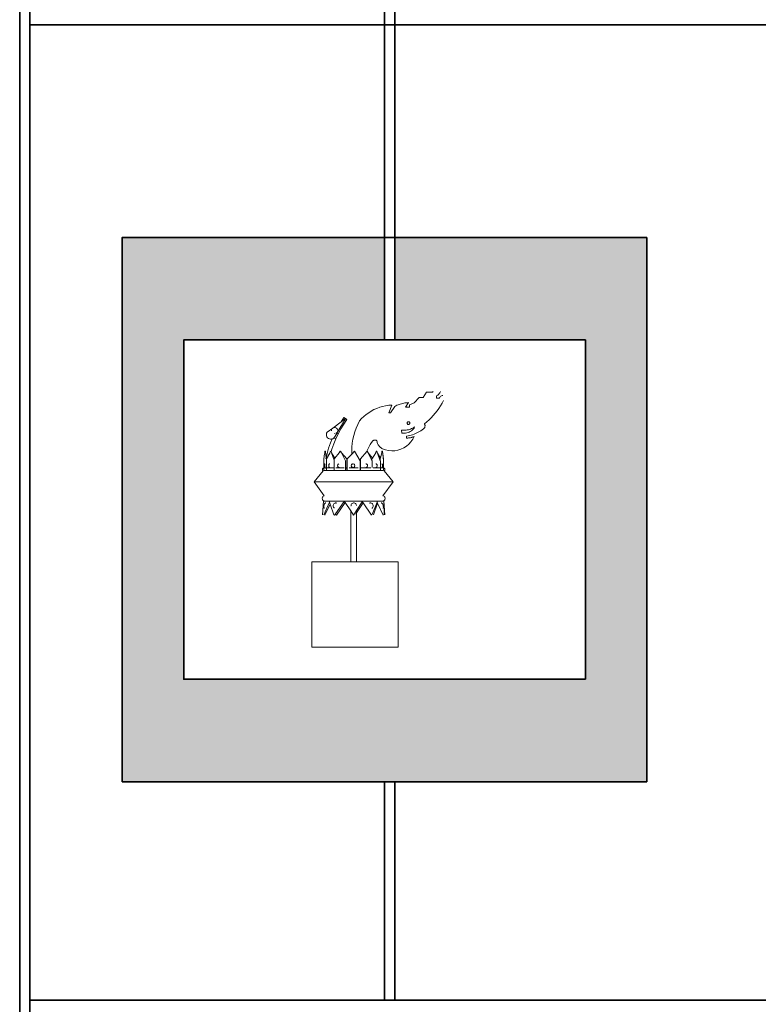
# Model space of a CAD drawing. Units: millimetres. Extents: x 2322 to 2394, y 1600 to 1790.
# Tile 2 of 5: x 2322 to 2358, y 1648 to 1696. Entities that reach past the tile are written whole.
import ezdxf

# ---------------------------------------------------------------- set-up
doc = ezdxf.new("R2010")
doc.units = ezdxf.units.MM
for name, color, linetype, lineweight in [('A-FURN', 7, 'Continuous', 35), ('A-FURN-ACCS', 8, 'Continuous', 18), ('A-FURN-PATT', 18, 'Continuous', 13)]:
    doc.layers.add(name, color=color, linetype=linetype, lineweight=lineweight)

msp = doc.modelspace()

# ---------------------------------------------------------------- hatches: boundary and pattern name
at = {"layer": 'A-FURN-PATT'}
h = msp.add_hatch(color=256, dxfattribs=at)
h.dxf.hatch_style = 1
h.paths.add_polyline_path([(2392.874, 1742.691), (2367.299, 1742.691), (2367.299, 1716.15), (2378.094, 1716.15), (2378.094, 1721.15), (2376.822, 1721.15), (2370.299, 1721.15), (2370.299, 1737.691), (2389.874, 1737.691), (2389.874, 1721.15), (2378.594, 1721.15), (2378.594, 1716.15), (2392.874, 1716.15)])
h.paths.add_polyline_path([(2352.154, 1685.571), (2339.867, 1685.571), (2339.867, 1680.571), (2349.154, 1680.571), (2349.154, 1664.029), (2329.579, 1664.029), (2329.579, 1680.571), (2339.367, 1680.571), (2339.367, 1685.571), (2326.579, 1685.571), (2326.579, 1659.029), (2352.154, 1659.029)])
h.paths.add_polyline_path([(2390.882, 1635.073), (2365.307, 1635.073), (2365.307, 1608.531), (2390.882, 1608.531)])
h.paths.add_polyline_path([(2387.882, 1630.073), (2387.882, 1613.531), (2368.307, 1613.531), (2368.307, 1630.073)], flags=16)
h.paths.add_polyline_path([(2373.463, 1622.711), (2373.46, 1622.644), (2373.462, 1622.642)], flags=0)
h.paths.add_polyline_path([(2380.387, 1618.619), (2380.387, 1618.619), (2380.35, 1618.619)], flags=0)
h.paths.add_polyline_path([(2377.431, 1618.132), (2377.363, 1618.141), (2377.19, 1618.152), (2377.145, 1618.149), (2376.982, 1618.132)], flags=0)
h.paths.add_polyline_path([(2376.126, 1618.152), (2375.767, 1618.152), (2375.734, 1618.152), (2375.734, 1618.152), (2375.028, 1618.152), (2375.028, 1618.198), (2374.578, 1618.295), (2374.235, 1618.449), (2373.926, 1618.69), (2373.709, 1619.163), (2373.66, 1619.336), (2373.672, 1619.402), (2373.73, 1620.54), (2373.702, 1622.038), (2373.678, 1622.131), (2373.705, 1621.917), (2373.73, 1620.54), (2373.667, 1619.311), (2373.709, 1619.163), (2373.87, 1618.812), (2373.949, 1618.699), (2374.037, 1618.604), (2374.187, 1618.486), (2374.3, 1618.42), (2374.485, 1618.337), (2374.688, 1618.272), (2374.979, 1618.209), (2375.028, 1618.203), (2375.028, 1618.372), (2375.028, 1618.619), (2377.125, 1618.619), (2377.165, 1620.356), (2377.172, 1620.356), (2377.172, 1620.357), (2377.341, 1620.357), (2377.354, 1620.357), (2377.354, 1623.532), (2377.38, 1623.766), (2377.629, 1623.72), (2377.726, 1623.72), (2377.722, 1623.891), (2377.719, 1624.041), (2377.644, 1624.123), (2377.631, 1624.228), (2377.644, 1624.211), (2377.677, 1624.213), (2377.688, 1624.153), (2377.757, 1624.059), (2377.78, 1623.72), (2377.883, 1623.72), (2378.152, 1623.76), (2378.155, 1620.358), (2378.298, 1620.356), (2378.301, 1620.356), (2378.362, 1620.357), (2378.402, 1618.619), (2377.354, 1618.619), (2377.125, 1618.619), (2375.028, 1618.619), (2375.028, 1618.372), (2375.028, 1618.177), (2375.049, 1618.152), (2375.734, 1618.152), (2375.756, 1618.153), (2375.767, 1618.152), (2376.126, 1618.152), (2376.144, 1618.154), (2376.168, 1618.151)], flags=0)
h.paths.add_polyline_path([(2380.5, 1618.343), (2380.401, 1618.342), (2380.5, 1618.342)], flags=0)
h.paths.add_polyline_path([(2378.836, 1627.111), (2378.86, 1627.114), (2378.771, 1627.114), (2378.773, 1627.108)], flags=0)
h.paths.add_polyline_path([(2378.972, 1627.091), (2379.09, 1626.957), (2378.972, 1626.879), (2378.964, 1626.862), (2378.975, 1626.787), (2379.128, 1626.434), (2379.25, 1626.246), (2379.42, 1626.03), (2379.646, 1625.791), (2380.15, 1625.354), (2380.519, 1624.956), (2380.743, 1624.553), (2380.884, 1624.119), (2380.94, 1623.673), (2380.977, 1621.652), (2380.892, 1619.98), (2380.807, 1619.502), (2380.712, 1619.163), (2380.621, 1618.942), (2380.422, 1618.619), (2380.413, 1618.619), (2380.386, 1618.619), (2380.474, 1618.703), (2380.621, 1618.942), (2380.712, 1619.163), (2380.807, 1619.502), (2380.892, 1619.98), (2380.977, 1621.652), (2380.94, 1623.673), (2380.9, 1623.987), (2380.843, 1624.244), (2380.778, 1624.446), (2380.693, 1624.644), (2380.585, 1624.839), (2380.452, 1625.029), (2380.15, 1625.354), (2379.646, 1625.791), (2379.324, 1626.132), (2379.128, 1626.434), (2378.92, 1626.915), (2378.841, 1626.975), (2378.869, 1626.811), (2379.027, 1626.915), (2379.041, 1626.939), (2379.037, 1626.997), (2379.02, 1627.036), (2378.879, 1627.196), (2378.841, 1627.151)], flags=0)
h.paths.add_polyline_path([(2375.501, 1627.114), (2375.642, 1627.103), (2375.561, 1626.855), (2375.555, 1626.827), (2375.48, 1626.868), (2375.292, 1626.434), (2375.097, 1626.132), (2374.775, 1625.791), (2374.271, 1625.354), (2374.13, 1625.216), (2373.969, 1625.029), (2373.836, 1624.839), (2373.728, 1624.644), (2373.643, 1624.446), (2373.537, 1624.119), (2373.52, 1623.987), (2373.601, 1624.348), (2373.773, 1624.748), (2374.034, 1625.122), (2374.271, 1625.354), (2374.775, 1625.791), (2375.001, 1626.03), (2375.171, 1626.246), (2375.292, 1626.434), (2375.445, 1626.787), (2375.447, 1626.797), (2375.334, 1627.042)], flags=0)
h.paths.add_polyline_path([(2375.398, 1627.114), (2375.384, 1626.997), (2375.411, 1627.054), (2375.531, 1627.169), (2375.597, 1627.114)], flags=0)
h.paths.add_polyline_path([(2377.985, 1623.628), (2377.785, 1623.645), (2377.786, 1623.634), (2377.764, 1623.634), (2377.729, 1623.636), (2377.728, 1623.656), (2377.701, 1623.664), (2377.421, 1623.752), (2377.412, 1623.748), (2377.629, 1623.72), (2377.78, 1623.72), (2377.783, 1623.68)], flags=0)
h.paths.add_polyline_path([(2377.348, 1620.357), (2377.335, 1620.357), (2377.327, 1620.356), (2377.354, 1620.356)], flags=0)
h.paths.add_polyline_path([(2377.834, 1620.357), (2377.854, 1620.356), (2377.911, 1620.356), (2377.923, 1620.357)], flags=0)
h.paths.add_polyline_path([(2378.155, 1620.356), (2378.155, 1620.356), (2378.014, 1620.356), (2378.002, 1620.357), (2377.96, 1620.356), (2377.956, 1620.356), (2377.923, 1620.357), (2378.111, 1620.357), (2378.119, 1620.356), (2378.144, 1620.356), (2378.163, 1620.357), (2378.163, 1620.357), (2378.157, 1620.357), (2378.149, 1620.356)], flags=0)
h.paths.add_polyline_path([(2377.609, 1620.357), (2377.623, 1620.356), (2377.653, 1620.357), (2377.738, 1620.356), (2377.743, 1620.357)], flags=0)
h.paths.add_polyline_path([(2380.479, 1618.152), (2380.406, 1618.152), (2380.313, 1618.151), (2380.107, 1618.152), (2380.104, 1618.152), (2380.108, 1618.151), (2379.961, 1618.152), (2379.793, 1618.152), (2377.32, 1618.152), (2377.3, 1618.149), (2377.253, 1618.152), (2379.793, 1618.152), (2380.01, 1618.153), (2380.21, 1618.152), (2380.229, 1618.152), (2380.231, 1618.152), (2380.394, 1618.152), (2380.48, 1618.152)], flags=0)

# ---------------------------------------------------------------- linework, layer by layer
at = {"layer": 'A-FURN'}
for p, q in [((2321.58, 1599.925), (2321.58, 1755.925)), ((2322.08, 1600.425), (2322.08, 1755.425)), ((2339.367, 1680.571), (2339.367, 1701.937)), ((2339.867, 1680.571), (2339.867, 1701.937)), ((2322.08, 1695.937), (2393.08, 1695.937)), ((2352.154, 1685.571), (2352.154, 1659.029)), ((2339.367, 1648.381), (2339.367, 1659.029)), ((2339.867, 1648.381), (2339.867, 1659.029)), ((2393.08, 1648.381), (2322.08, 1648.381))]:
    msp.add_line(p, q, dxfattribs=at)
msp.add_lwpolyline([(2352.154, 1659.029), (2326.579, 1659.029), (2326.579, 1685.571), (2352.154, 1685.571)], dxfattribs=at)
msp.add_lwpolyline([(2349.154, 1664.029), (2329.579, 1664.029), (2329.579, 1680.571), (2349.154, 1680.571)], close=True, dxfattribs=at)
at = {"layer": 'A-FURN-ACCS'}
for p, q in [((2341.248, 1677.774), (2341.407, 1678.032)), ((2341.407, 1678.032), (2341.702, 1678.032)), ((2341.702, 1678.032), (2341.729, 1678.056)), ((2341.931, 1677.862), (2341.9, 1677.844)), ((2341.9, 1677.844), (2341.9, 1677.731)), ((2341.96, 1677.883), (2341.931, 1677.862)), ((2341.987, 1677.906), (2341.96, 1677.883)), ((2342.011, 1677.931), (2341.987, 1677.906)), ((2342.033, 1677.959), (2342.011, 1677.931)), ((2342.053, 1677.989), (2342.033, 1677.959)), ((2342.069, 1678.021), (2342.053, 1677.989)), ((2342.083, 1678.053), (2342.069, 1678.021)), ((2342.088, 1677.805), (2342.113, 1677.826)), ((2342.113, 1677.826), (2342.139, 1677.844)), ((2342.139, 1677.844), (2342.168, 1677.859)), ((2342.168, 1677.859), (2342.198, 1677.871)), ((2339.27, 1677.331), (2339.416, 1677.364)), ((2339.416, 1677.364), (2339.565, 1677.387)), ((2339.565, 1677.387), (2339.714, 1677.399)), ((2339.714, 1677.399), (2339.567, 1677.027)), ((2339.66, 1677.027), (2339.857, 1677.336)), ((2339.857, 1677.336), (2339.91, 1677.362)), ((2339.91, 1677.362), (2339.964, 1677.386)), ((2339.964, 1677.386), (2340.019, 1677.408)), ((2340.019, 1677.408), (2340.074, 1677.428)), ((2340.074, 1677.428), (2340.13, 1677.446)), ((2340.13, 1677.446), (2340.187, 1677.462)), ((2340.187, 1677.462), (2340.244, 1677.477)), ((2340.244, 1677.477), (2340.302, 1677.489)), ((2340.302, 1677.489), (2340.36, 1677.499)), ((2340.36, 1677.499), (2340.419, 1677.506)), ((2340.536, 1677.516), (2340.391, 1677.289)), ((2340.419, 1677.506), (2340.478, 1677.512)), ((2340.478, 1677.512), (2340.536, 1677.516)), ((2340.585, 1677.415), (2340.8, 1677.501)), ((2340.585, 1677.289), (2340.585, 1677.415)), ((2340.8, 1677.501), (2341.05, 1677.774)), ((2341.05, 1677.774), (2341.248, 1677.774)), ((2341.9, 1677.731), (2342.026, 1677.731)), ((2342.092, 1677.362), (2342.011, 1677.238)), ((2342.026, 1677.731), (2342.044, 1677.757)), ((2342.044, 1677.757), (2342.065, 1677.782)), ((2342.065, 1677.782), (2342.088, 1677.805)), ((2342.167, 1677.489), (2342.092, 1677.362)), ((2342.236, 1677.619), (2342.167, 1677.489)), ((2338.354, 1676.84), (2338.469, 1676.936)), ((2338.469, 1676.936), (2338.59, 1677.024)), ((2338.59, 1677.024), (2338.717, 1677.104)), ((2338.717, 1677.104), (2338.849, 1677.174)), ((2338.849, 1677.174), (2338.986, 1677.236)), ((2338.986, 1677.236), (2339.126, 1677.288)), ((2339.126, 1677.288), (2339.27, 1677.331)), ((2339.567, 1677.027), (2339.66, 1677.027)), ((2340.391, 1677.289), (2340.585, 1677.289)), ((2341.737, 1676.89), (2341.636, 1676.783)), ((2341.834, 1677.002), (2341.737, 1676.89)), ((2341.925, 1677.118), (2341.834, 1677.002)), ((2342.011, 1677.238), (2341.925, 1677.118)), ((2337.246, 1676.583), (2336.842, 1676.278)), ((2337.456, 1676.729), (2337.044, 1676.028)), ((2337.231, 1676.236), (2337.371, 1676.467)), ((2337.386, 1676.787), (2337.246, 1676.583)), ((2337.456, 1676.74), (2337.246, 1676.583)), ((2337.371, 1676.467), (2337.525, 1676.692)), ((2337.456, 1676.74), (2337.386, 1676.787)), ((2337.456, 1676.729), (2337.456, 1676.74)), ((2337.525, 1676.692), (2337.456, 1676.74)), ((2338.058, 1676.454), (2337.982, 1676.279)), ((2338.144, 1676.625), (2338.058, 1676.454)), ((2338.144, 1676.625), (2338.245, 1676.736)), ((2338.245, 1676.736), (2338.354, 1676.84)), ((2340.462, 1676.529), (2340.466, 1676.546)), ((2340.462, 1676.512), (2340.462, 1676.529)), ((2340.466, 1676.495), (2340.462, 1676.512)), ((2340.466, 1676.546), (2340.475, 1676.561)), ((2340.475, 1676.479), (2340.466, 1676.495)), ((2340.475, 1676.561), (2340.488, 1676.574)), ((2340.487, 1676.467), (2340.475, 1676.479)), ((2340.502, 1676.458), (2340.487, 1676.467)), ((2340.488, 1676.574), (2340.503, 1676.582)), ((2340.519, 1676.453), (2340.502, 1676.458)), ((2340.503, 1676.582), (2340.52, 1676.587)), ((2340.537, 1676.453), (2340.519, 1676.453)), ((2340.52, 1676.587), (2340.538, 1676.587)), ((2340.554, 1676.458), (2340.537, 1676.453)), ((2340.538, 1676.587), (2340.555, 1676.582)), ((2340.569, 1676.467), (2340.554, 1676.458)), ((2340.555, 1676.582), (2340.57, 1676.573)), ((2340.582, 1676.479), (2340.569, 1676.467)), ((2340.57, 1676.573), (2340.582, 1676.561)), ((2340.582, 1676.561), (2340.591, 1676.546)), ((2340.591, 1676.494), (2340.582, 1676.479)), ((2340.591, 1676.546), (2340.595, 1676.529)), ((2340.595, 1676.511), (2340.591, 1676.494)), ((2340.595, 1676.529), (2340.595, 1676.511)), ((2341.42, 1676.582), (2341.305, 1676.489)), ((2341.305, 1676.489), (2341.317, 1676.469)), ((2341.317, 1676.469), (2341.326, 1676.447)), ((2341.326, 1676.447), (2341.332, 1676.425)), ((2341.332, 1676.425), (2341.336, 1676.401)), ((2341.336, 1676.378), (2341.334, 1676.354)), ((2341.336, 1676.401), (2341.336, 1676.378)), ((2341.53, 1676.68), (2341.42, 1676.582)), ((2341.636, 1676.783), (2341.53, 1676.68)), ((2336.539, 1676.023), (2336.529, 1675.969)), ((2336.529, 1675.958), (2336.529, 1675.969)), ((2336.529, 1675.958), (2336.533, 1675.903)), ((2336.533, 1675.903), (2336.552, 1675.851)), ((2336.564, 1676.073), (2336.539, 1676.023)), ((2336.842, 1676.278), (2336.564, 1676.073)), ((2336.778, 1676.15), (2336.78, 1676.187)), ((2336.778, 1676.149), (2336.778, 1676.15)), ((2336.778, 1676.143), (2336.778, 1676.149)), ((2336.78, 1676.187), (2336.792, 1676.222)), ((2336.792, 1676.222), (2336.813, 1676.253)), ((2336.813, 1676.253), (2336.842, 1676.278)), ((2336.842, 1676.278), (2336.876, 1676.295)), ((2336.876, 1676.295), (2336.913, 1676.303)), ((2336.913, 1676.303), (2336.952, 1676.301)), ((2336.927, 1676.02), (2336.924, 1676.013)), ((2337.039, 1676.018), (2336.929, 1675.831)), ((2336.952, 1676.301), (2336.988, 1676.289)), ((2336.988, 1676.289), (2337.021, 1676.269)), ((2336.989, 1675.755), (2337.099, 1675.989)), ((2336.996, 1676.038), (2337.003, 1676.034)), ((2337.015, 1676.043), (2337.01, 1676.045)), ((2337.021, 1676.269), (2337.046, 1676.242)), ((2337.044, 1676.028), (2337.039, 1676.018)), ((2337.099, 1675.989), (2337.039, 1676.018)), ((2337.044, 1676.028), (2337.103, 1675.998)), ((2337.046, 1676.242), (2337.064, 1676.208)), ((2337.064, 1676.208), (2337.072, 1676.172)), ((2337.071, 1676.167), (2337.072, 1676.172)), ((2337.071, 1676.167), (2337.072, 1676.166)), ((2337.231, 1676.236), (2337.103, 1675.998)), ((2337.865, 1675.915), (2337.823, 1675.729)), ((2337.918, 1676.099), (2337.865, 1675.915)), ((2337.982, 1676.279), (2337.918, 1676.099)), ((2340.245, 1676.169), (2340.189, 1676.174)), ((2340.189, 1676.174), (2340.203, 1676.034)), ((2340.264, 1676.025), (2340.203, 1676.034)), ((2340.302, 1676.167), (2340.245, 1676.169)), ((2340.326, 1676.023), (2340.264, 1676.025)), ((2340.358, 1676.169), (2340.302, 1676.167)), ((2340.388, 1676.028), (2340.326, 1676.023)), ((2340.414, 1676.174), (2340.358, 1676.169)), ((2340.449, 1676.038), (2340.388, 1676.028)), ((2340.469, 1676.183), (2340.414, 1676.174)), ((2340.51, 1675.895), (2340.435, 1675.882)), ((2340.508, 1676.056), (2340.449, 1676.038)), ((2340.524, 1676.194), (2340.469, 1676.183)), ((2340.566, 1676.079), (2340.508, 1676.056)), ((2340.584, 1675.911), (2340.51, 1675.895)), ((2340.578, 1676.209), (2340.524, 1676.194)), ((2340.62, 1676.108), (2340.566, 1676.079)), ((2340.632, 1676.227), (2340.578, 1676.209)), ((2340.657, 1675.931), (2340.584, 1675.911)), ((2340.671, 1676.143), (2340.62, 1676.108)), ((2340.684, 1676.248), (2340.632, 1676.227)), ((2340.73, 1675.953), (2340.657, 1675.931)), ((2340.718, 1676.183), (2340.671, 1676.143)), ((2340.735, 1676.272), (2340.684, 1676.248)), ((2340.761, 1676.228), (2340.718, 1676.183)), ((2340.801, 1675.978), (2340.73, 1675.953)), ((2340.784, 1676.3), (2340.735, 1676.272)), ((2340.799, 1676.277), (2340.761, 1676.228)), ((2340.831, 1676.33), (2340.784, 1676.3)), ((2340.831, 1676.33), (2340.799, 1676.277)), ((2340.871, 1676.007), (2340.801, 1675.978)), ((2340.941, 1676.038), (2340.871, 1676.007)), ((2341.008, 1676.072), (2340.941, 1676.038)), ((2341.074, 1676.109), (2341.008, 1676.072)), ((2341.139, 1676.149), (2341.074, 1676.109)), ((2341.202, 1676.191), (2341.139, 1676.149)), ((2341.263, 1676.236), (2341.202, 1676.191)), ((2341.281, 1676.252), (2341.263, 1676.236)), ((2341.296, 1676.269), (2341.281, 1676.252)), ((2341.31, 1676.288), (2341.296, 1676.269)), ((2341.32, 1676.309), (2341.31, 1676.288)), ((2341.329, 1676.331), (2341.32, 1676.309)), ((2341.334, 1676.354), (2341.329, 1676.331)), ((2336.552, 1675.851), (2336.584, 1675.806)), ((2336.584, 1675.806), (2336.627, 1675.77)), ((2336.627, 1675.77), (2336.678, 1675.746)), ((2336.729, 1675.562), (2336.639, 1675.298)), ((2336.678, 1675.746), (2336.734, 1675.736)), ((2336.803, 1675.744), (2336.729, 1675.562)), ((2336.734, 1675.736), (2336.791, 1675.74)), ((2336.791, 1675.74), (2336.803, 1675.744)), ((2336.799, 1675.248), (2336.887, 1675.503)), ((2336.803, 1675.744), (2336.845, 1675.758)), ((2336.808, 1675.756), (2336.803, 1675.744)), ((2336.845, 1675.758), (2336.892, 1675.789)), ((2336.887, 1675.503), (2336.988, 1675.754)), ((2336.888, 1675.797), (2336.896, 1675.794)), ((2336.892, 1675.789), (2336.896, 1675.794)), ((2336.899, 1675.797), (2336.893, 1675.8)), ((2336.896, 1675.794), (2336.899, 1675.797)), ((2336.896, 1675.794), (2336.988, 1675.754)), ((2336.899, 1675.797), (2336.929, 1675.831)), ((2336.899, 1675.797), (2336.989, 1675.755)), ((2336.913, 1675.791), (2336.911, 1675.787)), ((2336.941, 1675.851), (2336.913, 1675.791)), ((2337.792, 1675.54), (2337.774, 1675.35)), ((2337.823, 1675.729), (2337.792, 1675.54)), ((2338.665, 1675.474), (2338.608, 1675.378)), ((2338.729, 1675.565), (2338.665, 1675.474)), ((2338.8, 1675.65), (2338.729, 1675.565)), ((2338.813, 1675.663), (2338.8, 1675.65)), ((2338.828, 1675.673), (2338.813, 1675.663)), ((2338.843, 1675.681), (2338.828, 1675.673)), ((2338.86, 1675.687), (2338.843, 1675.681)), ((2338.877, 1675.691), (2338.86, 1675.687)), ((2338.895, 1675.692), (2338.877, 1675.691)), ((2338.913, 1675.691), (2338.895, 1675.692)), ((2338.93, 1675.687), (2338.913, 1675.691)), ((2338.947, 1675.681), (2338.93, 1675.687)), ((2338.963, 1675.673), (2338.947, 1675.681)), ((2338.977, 1675.663), (2338.963, 1675.673)), ((2338.99, 1675.65), (2338.977, 1675.663)), ((2338.996, 1675.609), (2338.99, 1675.65)), ((2339.006, 1675.569), (2338.996, 1675.609)), ((2339.019, 1675.53), (2339.006, 1675.569)), ((2339.035, 1675.492), (2339.019, 1675.53)), ((2339.055, 1675.455), (2339.035, 1675.492)), ((2339.078, 1675.42), (2339.055, 1675.455)), ((2339.104, 1675.388), (2339.078, 1675.42)), ((2340.546, 1675.489), (2340.43, 1675.39)), ((2340.435, 1675.882), (2340.435, 1675.785)), ((2340.435, 1675.785), (2340.467, 1675.787)), ((2340.467, 1675.787), (2340.498, 1675.789)), ((2340.498, 1675.789), (2340.53, 1675.793)), ((2340.53, 1675.793), (2340.561, 1675.797)), ((2340.649, 1675.602), (2340.546, 1675.489)), ((2340.561, 1675.797), (2340.593, 1675.802)), ((2340.593, 1675.802), (2340.624, 1675.808)), ((2340.624, 1675.808), (2340.655, 1675.815)), ((2340.736, 1675.728), (2340.649, 1675.602)), ((2340.655, 1675.815), (2340.685, 1675.823)), ((2340.685, 1675.823), (2340.716, 1675.832)), ((2340.716, 1675.832), (2340.746, 1675.842)), ((2340.806, 1675.864), (2340.736, 1675.728)), ((2340.746, 1675.842), (2340.776, 1675.852)), ((2340.776, 1675.852), (2340.806, 1675.864)), ((2336.443, 1675.02), (2336.398, 1674.769)), ((2336.443, 1675.02), (2336.446, 1675.046)), ((2336.446, 1675.046), (2336.459, 1675.151)), ((2336.466, 1675.151), (2336.446, 1675.046)), ((2336.466, 1675.151), (2336.459, 1675.151)), ((2336.466, 1675.151), (2336.483, 1675.151)), ((2336.489, 1675.091), (2336.483, 1675.151)), ((2336.489, 1675.091), (2336.532, 1674.894)), ((2336.516, 1674.826), (2336.489, 1675.091)), ((2336.693, 1675.06), (2336.527, 1674.769)), ((2336.562, 1675.029), (2336.532, 1674.894)), ((2336.639, 1675.298), (2336.562, 1675.029)), ((2336.644, 1675.008), (2336.631, 1674.952)), ((2336.693, 1675.06), (2336.724, 1675.151)), ((2336.744, 1675.151), (2336.693, 1675.06)), ((2336.728, 1675.151), (2336.724, 1675.151)), ((2336.757, 1675.151), (2336.744, 1675.151)), ((2336.765, 1675.127), (2336.757, 1675.151)), ((2336.765, 1675.127), (2336.799, 1675.248)), ((2336.782, 1675.075), (2336.765, 1675.127)), ((2336.782, 1675.075), (2336.94, 1674.813)), ((2336.903, 1674.708), (2336.782, 1675.075)), ((2337.15, 1675.066), (2336.94, 1674.813)), ((2337.15, 1675.066), (2337.192, 1675.151)), ((2337.21, 1675.138), (2337.15, 1675.066)), ((2337.199, 1675.151), (2337.192, 1675.151)), ((2337.199, 1675.151), (2337.21, 1675.138)), ((2337.221, 1675.151), (2337.21, 1675.138)), ((2337.229, 1675.151), (2337.221, 1675.151)), ((2337.267, 1675.071), (2337.229, 1675.151)), ((2337.249, 1675.093), (2337.267, 1675.071)), ((2337.267, 1675.071), (2337.525, 1674.769)), ((2337.46, 1674.671), (2337.267, 1675.071)), ((2337.771, 1675.009), (2337.543, 1674.769)), ((2337.774, 1675.35), (2337.767, 1675.159)), ((2337.767, 1675.159), (2337.771, 1675.009)), ((2337.905, 1675.151), (2337.771, 1675.009)), ((2338.168, 1674.671), (2337.905, 1675.151)), ((2338.506, 1675.137), (2338.19, 1674.769)), ((2338.506, 1675.137), (2338.503, 1675.127)), ((2338.507, 1675.14), (2338.506, 1675.137)), ((2338.506, 1675.137), (2338.509, 1675.134)), ((2338.517, 1675.175), (2338.507, 1675.14)), ((2338.516, 1675.151), (2338.507, 1675.14)), ((2338.516, 1675.151), (2338.523, 1675.151)), ((2338.559, 1675.278), (2338.517, 1675.175)), ((2338.565, 1675.066), (2338.523, 1675.151)), ((2338.608, 1675.378), (2338.559, 1675.278)), ((2338.565, 1675.066), (2338.776, 1674.813)), ((2338.565, 1675.066), (2338.749, 1674.693)), ((2338.933, 1675.075), (2338.776, 1674.813)), ((2338.933, 1675.075), (2338.958, 1675.151)), ((2338.975, 1675.145), (2338.933, 1675.075)), ((2338.958, 1675.151), (2338.971, 1675.151)), ((2338.971, 1675.151), (2338.975, 1675.145)), ((2338.978, 1675.151), (2338.975, 1675.145)), ((2338.978, 1675.151), (2338.991, 1675.151)), ((2339.023, 1675.06), (2338.991, 1675.151)), ((2339.023, 1675.06), (2339.165, 1674.81)), ((2339.023, 1675.06), (2339.156, 1674.677)), ((2339.132, 1675.358), (2339.104, 1675.388)), ((2339.163, 1675.33), (2339.132, 1675.358)), ((2339.196, 1675.306), (2339.163, 1675.33)), ((2339.226, 1675.091), (2339.165, 1674.81)), ((2339.232, 1675.284), (2339.196, 1675.306)), ((2339.226, 1675.091), (2339.233, 1675.151)), ((2339.239, 1675.151), (2339.226, 1675.091)), ((2339.269, 1675.265), (2339.232, 1675.284)), ((2339.233, 1675.151), (2339.239, 1675.151)), ((2339.239, 1675.151), (2339.256, 1675.151)), ((2339.256, 1675.151), (2339.273, 1675.02)), ((2339.412, 1675.212), (2339.269, 1675.265)), ((2339.273, 1675.02), (2339.317, 1674.769)), ((2339.317, 1674.671), (2339.273, 1675.02)), ((2339.561, 1675.178), (2339.412, 1675.212)), ((2339.713, 1675.165), (2339.561, 1675.178)), ((2339.866, 1675.171), (2339.713, 1675.165)), ((2340.017, 1675.197), (2339.866, 1675.171)), ((2340.162, 1675.243), (2340.017, 1675.197)), ((2340.301, 1675.308), (2340.162, 1675.243)), ((2340.43, 1675.39), (2340.301, 1675.308)), ((2336.398, 1674.769), (2336.399, 1674.677)), ((2336.398, 1674.671), (2336.399, 1674.677)), ((2336.398, 1674.671), (2336.398, 1674.329)), ((2336.427, 1674.456), (2336.428, 1674.477)), ((2336.427, 1674.434), (2336.427, 1674.456)), ((2336.428, 1674.477), (2336.431, 1674.496)), ((2336.431, 1674.496), (2336.433, 1674.512)), ((2336.433, 1674.512), (2336.437, 1674.523)), ((2336.436, 1674.456), (2336.437, 1674.477)), ((2336.436, 1674.434), (2336.436, 1674.456)), ((2336.437, 1674.523), (2336.441, 1674.528)), ((2336.437, 1674.477), (2336.439, 1674.496)), ((2336.439, 1674.496), (2336.442, 1674.512)), ((2336.449, 1674.528), (2336.441, 1674.528)), ((2336.442, 1674.512), (2336.445, 1674.523)), ((2336.445, 1674.523), (2336.449, 1674.528)), ((2336.451, 1674.477), (2336.45, 1674.456)), ((2336.45, 1674.456), (2336.45, 1674.434)), ((2336.454, 1674.496), (2336.451, 1674.477)), ((2336.454, 1674.481), (2336.451, 1674.477)), ((2336.457, 1674.512), (2336.454, 1674.496)), ((2336.454, 1674.496), (2336.454, 1674.481)), ((2336.459, 1674.517), (2336.457, 1674.512)), ((2336.46, 1674.515), (2336.457, 1674.512)), ((2336.459, 1674.477), (2336.458, 1674.456)), ((2336.458, 1674.456), (2336.458, 1674.434)), ((2336.462, 1674.496), (2336.459, 1674.477)), ((2336.463, 1674.501), (2336.462, 1674.496)), ((2336.516, 1674.826), (2336.505, 1674.776)), ((2336.532, 1674.894), (2336.516, 1674.826)), ((2336.527, 1674.719), (2336.516, 1674.826)), ((2336.527, 1674.769), (2336.527, 1674.719)), ((2336.527, 1674.719), (2336.527, 1674.33)), ((2336.532, 1674.894), (2336.544, 1674.838)), ((2336.641, 1674.456), (2336.644, 1674.477)), ((2336.641, 1674.434), (2336.641, 1674.456)), ((2336.644, 1674.477), (2336.651, 1674.496)), ((2336.651, 1674.496), (2336.66, 1674.512)), ((2336.66, 1674.512), (2336.671, 1674.523)), ((2336.671, 1674.523), (2336.684, 1674.528)), ((2336.691, 1674.528), (2336.684, 1674.528)), ((2336.94, 1674.813), (2336.903, 1674.769)), ((2336.903, 1674.769), (2336.903, 1674.708)), ((2336.903, 1674.708), (2336.903, 1674.325)), ((2337.075, 1674.456), (2337.08, 1674.477)), ((2337.075, 1674.434), (2337.075, 1674.456)), ((2337.08, 1674.477), (2337.09, 1674.496)), ((2337.09, 1674.496), (2337.103, 1674.512)), ((2337.103, 1674.512), (2337.12, 1674.523)), ((2337.12, 1674.523), (2337.139, 1674.528)), ((2337.143, 1674.528), (2337.139, 1674.528)), ((2337.46, 1674.671), (2337.463, 1674.33)), ((2337.525, 1674.769), (2337.525, 1674.33)), ((2337.543, 1674.769), (2337.543, 1674.33)), ((2337.743, 1674.456), (2337.749, 1674.477)), ((2337.743, 1674.434), (2337.743, 1674.456)), ((2337.749, 1674.477), (2337.76, 1674.496)), ((2337.76, 1674.496), (2337.776, 1674.512)), ((2337.776, 1674.512), (2337.795, 1674.523)), ((2337.795, 1674.523), (2337.816, 1674.528)), ((2337.816, 1674.528), (2337.838, 1674.528)), ((2337.838, 1674.528), (2337.859, 1674.523)), ((2337.859, 1674.523), (2337.878, 1674.512)), ((2337.878, 1674.512), (2337.894, 1674.496)), ((2337.894, 1674.496), (2337.905, 1674.477)), ((2337.905, 1674.477), (2337.91, 1674.456)), ((2337.91, 1674.456), (2337.91, 1674.434)), ((2338.168, 1674.671), (2338.17, 1674.404)), ((2338.19, 1674.769), (2338.19, 1674.404)), ((2338.443, 1674.528), (2338.447, 1674.528)), ((2338.447, 1674.528), (2338.467, 1674.528)), ((2338.467, 1674.528), (2338.486, 1674.523)), ((2338.486, 1674.523), (2338.503, 1674.512)), ((2338.503, 1674.512), (2338.517, 1674.496)), ((2338.517, 1674.496), (2338.527, 1674.477)), ((2338.527, 1674.477), (2338.532, 1674.456)), ((2338.532, 1674.456), (2338.532, 1674.434)), ((2338.776, 1674.813), (2338.749, 1674.769)), ((2338.749, 1674.769), (2338.749, 1674.693)), ((2338.76, 1674.671), (2338.749, 1674.693)), ((2338.76, 1674.671), (2338.762, 1674.355)), ((2338.935, 1674.528), (2338.941, 1674.528)), ((2338.941, 1674.528), (2338.955, 1674.528)), ((2338.955, 1674.528), (2338.969, 1674.523)), ((2338.969, 1674.523), (2338.981, 1674.512)), ((2338.981, 1674.512), (2338.991, 1674.496)), ((2338.991, 1674.496), (2338.998, 1674.477)), ((2338.998, 1674.477), (2339.001, 1674.456)), ((2339.001, 1674.456), (2339.001, 1674.434)), ((2339.165, 1674.81), (2339.156, 1674.769)), ((2339.156, 1674.769), (2339.156, 1674.677)), ((2339.158, 1674.671), (2339.156, 1674.677)), ((2339.158, 1674.671), (2339.16, 1674.33)), ((2339.235, 1674.528), (2339.24, 1674.528)), ((2339.24, 1674.528), (2339.245, 1674.523)), ((2339.24, 1674.528), (2339.243, 1674.528)), ((2339.243, 1674.528), (2339.249, 1674.528)), ((2339.245, 1674.523), (2339.25, 1674.512)), ((2339.249, 1674.528), (2339.253, 1674.523)), ((2339.25, 1674.512), (2339.253, 1674.496)), ((2339.253, 1674.523), (2339.258, 1674.512)), ((2339.253, 1674.496), (2339.256, 1674.477)), ((2339.256, 1674.477), (2339.257, 1674.456)), ((2339.257, 1674.456), (2339.257, 1674.434)), ((2339.258, 1674.512), (2339.261, 1674.496)), ((2339.261, 1674.496), (2339.264, 1674.477)), ((2339.264, 1674.477), (2339.265, 1674.456)), ((2339.265, 1674.456), (2339.265, 1674.434)), ((2339.317, 1674.769), (2339.317, 1674.671)), ((2339.317, 1674.671), (2339.317, 1674.329)), ((2335.929, 1673.648), (2336.365, 1674.199)), ((2336.337, 1674.248), (2336.338, 1674.267)), ((2336.342, 1674.229), (2336.337, 1674.248)), ((2336.338, 1674.267), (2336.343, 1674.286)), ((2336.352, 1674.213), (2336.342, 1674.229)), ((2336.343, 1674.286), (2336.353, 1674.302)), ((2336.365, 1674.199), (2336.352, 1674.213)), ((2336.353, 1674.302), (2336.367, 1674.316)), ((2336.367, 1674.316), (2336.383, 1674.325)), ((2336.383, 1674.325), (2336.398, 1674.329)), ((2336.398, 1674.229), (2336.397, 1674.213)), ((2336.399, 1674.213), (2336.397, 1674.213)), ((2336.423, 1674.213), (2336.397, 1674.213)), ((2336.398, 1674.329), (2336.402, 1674.33)), ((2336.398, 1674.329), (2336.398, 1674.325)), ((2336.398, 1674.316), (2336.398, 1674.248)), ((2336.402, 1674.33), (2336.405, 1674.33)), ((2336.402, 1674.33), (2336.403, 1674.33)), ((2336.501, 1674.33), (2336.405, 1674.33)), ((2336.423, 1674.213), (2336.422, 1674.204)), ((2336.422, 1674.204), (2336.422, 1674.199)), ((2336.527, 1674.213), (2336.423, 1674.213)), ((2336.428, 1674.413), (2336.427, 1674.434)), ((2336.43, 1674.394), (2336.428, 1674.413)), ((2336.433, 1674.378), (2336.43, 1674.394)), ((2336.437, 1674.367), (2336.433, 1674.378)), ((2336.437, 1674.413), (2336.436, 1674.434)), ((2336.439, 1674.394), (2336.437, 1674.413)), ((2336.441, 1674.361), (2336.437, 1674.367)), ((2336.442, 1674.378), (2336.439, 1674.394)), ((2336.445, 1674.361), (2336.441, 1674.361)), ((2336.45, 1674.434), (2336.442, 1674.378)), ((2336.445, 1674.367), (2336.442, 1674.378)), ((2336.449, 1674.361), (2336.445, 1674.367)), ((2336.449, 1674.361), (2336.445, 1674.361)), ((2336.453, 1674.361), (2336.449, 1674.361)), ((2336.45, 1674.434), (2336.451, 1674.412)), ((2336.451, 1674.412), (2336.454, 1674.393)), ((2336.454, 1674.393), (2336.457, 1674.378)), ((2336.457, 1674.378), (2336.459, 1674.373)), ((2336.458, 1674.434), (2336.459, 1674.412)), ((2336.459, 1674.412), (2336.462, 1674.393)), ((2336.462, 1674.393), (2336.463, 1674.389)), ((2336.508, 1674.213), (2336.506, 1674.199)), ((2336.527, 1674.33), (2336.516, 1674.33)), ((2336.527, 1674.314), (2336.516, 1674.314)), ((2336.52, 1674.316), (2336.517, 1674.287)), ((2336.527, 1674.382), (2336.521, 1674.325)), ((2336.527, 1674.33), (2336.527, 1674.325)), ((2336.527, 1674.316), (2336.527, 1674.314)), ((2336.527, 1674.314), (2336.527, 1674.248)), ((2336.527, 1674.229), (2336.527, 1674.213)), ((2336.527, 1674.213), (2336.593, 1674.213)), ((2336.871, 1674.33), (2336.567, 1674.33)), ((2336.591, 1674.199), (2336.593, 1674.213)), ((2336.593, 1674.213), (2336.904, 1674.213)), ((2336.644, 1674.413), (2336.641, 1674.434)), ((2336.65, 1674.394), (2336.644, 1674.413)), ((2336.66, 1674.378), (2336.65, 1674.394)), ((2336.671, 1674.367), (2336.66, 1674.378)), ((2336.684, 1674.361), (2336.671, 1674.367)), ((2336.697, 1674.361), (2336.684, 1674.361)), ((2336.704, 1674.361), (2336.697, 1674.361)), ((2336.903, 1674.316), (2336.903, 1674.248)), ((2336.903, 1674.229), (2336.904, 1674.213)), ((2336.904, 1674.213), (2337.464, 1674.213)), ((2336.985, 1674.33), (2337.389, 1674.33)), ((2337.08, 1674.413), (2337.075, 1674.434)), ((2337.089, 1674.394), (2337.08, 1674.413)), ((2337.103, 1674.378), (2337.089, 1674.394)), ((2337.12, 1674.367), (2337.103, 1674.378)), ((2337.138, 1674.361), (2337.12, 1674.367)), ((2337.158, 1674.361), (2337.138, 1674.361)), ((2337.162, 1674.361), (2337.158, 1674.361)), ((2337.463, 1674.33), (2337.455, 1674.33)), ((2337.463, 1674.314), (2337.455, 1674.314)), ((2337.463, 1674.33), (2337.463, 1674.325)), ((2337.525, 1674.33), (2337.463, 1674.33)), ((2337.463, 1674.316), (2337.463, 1674.314)), ((2337.463, 1674.314), (2337.463, 1674.248)), ((2337.525, 1674.314), (2337.463, 1674.314)), ((2337.464, 1674.229), (2337.464, 1674.213)), ((2337.525, 1674.213), (2337.464, 1674.213)), ((2337.525, 1674.33), (2337.543, 1674.33)), ((2337.525, 1674.33), (2337.525, 1674.325)), ((2337.525, 1674.316), (2337.525, 1674.314)), ((2337.525, 1674.314), (2337.525, 1674.248)), ((2337.543, 1674.314), (2337.525, 1674.314)), ((2337.525, 1674.229), (2337.525, 1674.213)), ((2337.543, 1674.33), (2337.543, 1674.325)), ((2337.543, 1674.316), (2337.543, 1674.314)), ((2337.543, 1674.314), (2337.543, 1674.248)), ((2337.543, 1674.229), (2337.543, 1674.213)), ((2337.543, 1674.213), (2338.172, 1674.213)), ((2337.634, 1674.33), (2338.081, 1674.33)), ((2337.749, 1674.413), (2337.743, 1674.434)), ((2337.76, 1674.394), (2337.749, 1674.413)), ((2337.775, 1674.378), (2337.76, 1674.394)), ((2337.794, 1674.367), (2337.775, 1674.378)), ((2337.816, 1674.361), (2337.794, 1674.367)), ((2337.838, 1674.361), (2337.816, 1674.361)), ((2337.859, 1674.367), (2337.838, 1674.361)), ((2337.878, 1674.378), (2337.859, 1674.367)), ((2337.893, 1674.393), (2337.878, 1674.378)), ((2337.904, 1674.412), (2337.893, 1674.393)), ((2337.91, 1674.434), (2337.904, 1674.412)), ((2338.19, 1674.404), (2338.17, 1674.404)), ((2338.17, 1674.404), (2338.171, 1674.33)), ((2338.171, 1674.33), (2338.171, 1674.325)), ((2338.19, 1674.33), (2338.171, 1674.33)), ((2338.171, 1674.316), (2338.171, 1674.314)), ((2338.171, 1674.314), (2338.172, 1674.248)), ((2338.19, 1674.314), (2338.171, 1674.314)), ((2338.172, 1674.229), (2338.172, 1674.213)), ((2338.19, 1674.213), (2338.172, 1674.213)), ((2338.198, 1674.404), (2338.19, 1674.404)), ((2338.19, 1674.404), (2338.19, 1674.33)), ((2338.198, 1674.33), (2338.19, 1674.33)), ((2338.19, 1674.33), (2338.19, 1674.325)), ((2338.19, 1674.316), (2338.19, 1674.314)), ((2338.198, 1674.314), (2338.19, 1674.314)), ((2338.19, 1674.314), (2338.19, 1674.248)), ((2338.19, 1674.229), (2338.19, 1674.213)), ((2339.16, 1674.213), (2338.19, 1674.213)), ((2338.224, 1674.33), (2338.687, 1674.33)), ((2338.39, 1674.406), (2338.387, 1674.406)), ((2338.463, 1674.361), (2338.466, 1674.361)), ((2338.485, 1674.367), (2338.466, 1674.361)), ((2338.502, 1674.378), (2338.485, 1674.367)), ((2338.516, 1674.393), (2338.502, 1674.378)), ((2338.526, 1674.412), (2338.516, 1674.393)), ((2338.532, 1674.434), (2338.526, 1674.412)), ((2339.132, 1674.33), (2338.81, 1674.33)), ((2338.949, 1674.361), (2338.955, 1674.361)), ((2338.968, 1674.367), (2338.955, 1674.361)), ((2338.981, 1674.378), (2338.968, 1674.367)), ((2338.99, 1674.393), (2338.981, 1674.378)), ((2338.997, 1674.412), (2338.99, 1674.393)), ((2339.001, 1674.434), (2338.997, 1674.412)), ((2339.172, 1674.33), (2339.16, 1674.33)), ((2339.16, 1674.33), (2339.16, 1674.325)), ((2339.16, 1674.316), (2339.16, 1674.314)), ((2339.172, 1674.314), (2339.16, 1674.314)), ((2339.16, 1674.314), (2339.16, 1674.248)), ((2339.16, 1674.229), (2339.16, 1674.213)), ((2339.317, 1674.213), (2339.16, 1674.213)), ((2339.194, 1674.33), (2339.3, 1674.33)), ((2339.245, 1674.367), (2339.24, 1674.361)), ((2339.24, 1674.361), (2339.248, 1674.361)), ((2339.25, 1674.378), (2339.245, 1674.367)), ((2339.253, 1674.367), (2339.248, 1674.361)), ((2339.253, 1674.393), (2339.25, 1674.378)), ((2339.256, 1674.412), (2339.253, 1674.393)), ((2339.258, 1674.378), (2339.253, 1674.367)), ((2339.257, 1674.434), (2339.256, 1674.412)), ((2339.261, 1674.393), (2339.258, 1674.378)), ((2339.264, 1674.412), (2339.261, 1674.393)), ((2339.265, 1674.434), (2339.264, 1674.412)), ((2339.317, 1674.329), (2339.332, 1674.325)), ((2339.317, 1674.329), (2339.317, 1674.325)), ((2339.317, 1674.316), (2339.317, 1674.248)), ((2339.317, 1674.229), (2339.317, 1674.213)), ((2339.332, 1674.325), (2339.349, 1674.316)), ((2339.349, 1674.316), (2339.362, 1674.302)), ((2339.364, 1674.213), (2339.35, 1674.199)), ((2339.35, 1674.199), (2339.786, 1673.648)), ((2339.362, 1674.302), (2339.372, 1674.286)), ((2339.373, 1674.229), (2339.364, 1674.213)), ((2339.372, 1674.286), (2339.377, 1674.267)), ((2339.378, 1674.248), (2339.373, 1674.229)), ((2339.377, 1674.267), (2339.378, 1674.248)), ((2336.428, 1672.98), (2335.929, 1673.648)), ((2339.786, 1673.648), (2335.929, 1673.648)), ((2339.786, 1673.648), (2339.287, 1672.98)), ((2336.324, 1672.836), (2336.325, 1672.869)), ((2336.332, 1672.805), (2336.324, 1672.836)), ((2336.325, 1672.869), (2336.333, 1672.9)), ((2336.346, 1672.776), (2336.332, 1672.805)), ((2336.333, 1672.9), (2336.349, 1672.928)), ((2336.342, 1672.047), (2336.388, 1672.718)), ((2336.368, 1672.752), (2336.346, 1672.776)), ((2336.349, 1672.928), (2336.371, 1672.952)), ((2336.394, 1672.734), (2336.368, 1672.752)), ((2336.371, 1672.952), (2336.398, 1672.97)), ((2336.456, 1672.718), (2336.388, 1672.718)), ((2336.424, 1672.722), (2336.394, 1672.734)), ((2336.398, 1672.97), (2336.428, 1672.98)), ((2336.402, 1672.045), (2336.678, 1672.66)), ((2336.415, 1672.52), (2336.426, 1672.552)), ((2336.456, 1672.718), (2336.424, 1672.722)), ((2336.426, 1672.552), (2336.439, 1672.581)), ((2336.439, 1672.581), (2336.452, 1672.604)), ((2336.446, 1672.032), (2336.71, 1672.568)), ((2336.452, 1672.604), (2336.465, 1672.621)), ((2336.456, 1672.718), (2336.644, 1672.718)), ((2336.465, 1672.621), (2336.477, 1672.628)), ((2336.477, 1672.628), (2336.487, 1672.627)), ((2336.489, 1672.625), (2336.487, 1672.627)), ((2336.489, 1672.625), (2336.499, 1672.624)), ((2336.644, 1672.718), (2336.657, 1672.718)), ((2336.658, 1672.714), (2336.644, 1672.718)), ((2336.658, 1672.714), (2336.657, 1672.718)), ((2336.657, 1672.718), (2337.36, 1672.718)), ((2336.678, 1672.66), (2336.658, 1672.714)), ((2336.71, 1672.568), (2336.678, 1672.66)), ((2336.896, 1672.047), (2336.71, 1672.568)), ((2336.866, 1672.52), (2336.88, 1672.552)), ((2336.88, 1672.552), (2336.899, 1672.581)), ((2336.899, 1672.581), (2336.923, 1672.604)), ((2336.923, 1672.604), (2336.95, 1672.621)), ((2336.95, 1672.621), (2336.979, 1672.628)), ((2336.974, 1672.095), (2337.394, 1672.703)), ((2336.979, 1672.628), (2337.007, 1672.627)), ((2337.007, 1672.627), (2337.033, 1672.617)), ((2337.025, 1672.032), (2337.451, 1672.648)), ((2337.033, 1672.617), (2337.039, 1672.614)), ((2337.36, 1672.718), (2337.416, 1672.718)), ((2337.394, 1672.703), (2337.36, 1672.718)), ((2337.416, 1672.703), (2337.416, 1672.718)), ((2338.22, 1672.718), (2337.416, 1672.718)), ((2337.451, 1672.648), (2337.416, 1672.703)), ((2337.715, 1672.244), (2337.451, 1672.648)), ((2337.729, 1672.52), (2337.74, 1672.552)), ((2337.74, 1672.552), (2337.758, 1672.581)), ((2337.758, 1672.581), (2337.783, 1672.604)), ((2337.783, 1672.604), (2337.814, 1672.621)), ((2337.814, 1672.621), (2337.849, 1672.628)), ((2337.849, 1672.628), (2337.884, 1672.627)), ((2337.884, 1672.627), (2337.917, 1672.618)), ((2337.917, 1672.618), (2337.947, 1672.6)), ((2337.947, 1672.6), (2337.971, 1672.575)), ((2337.971, 1672.575), (2337.988, 1672.545)), ((2337.988, 1672.545), (2337.996, 1672.512)), ((2338.001, 1672.254), (2338.28, 1672.673)), ((2338.001, 1672.136), (2338.313, 1672.625)), ((2338.291, 1672.717), (2338.22, 1672.718)), ((2338.28, 1672.673), (2338.275, 1672.681)), ((2338.313, 1672.625), (2338.28, 1672.673)), ((2338.291, 1672.717), (2338.292, 1672.718)), ((2338.292, 1672.718), (2338.295, 1672.718)), ((2339.019, 1672.718), (2338.295, 1672.718)), ((2338.721, 1672.032), (2338.313, 1672.625)), ((2338.635, 1672.617), (2338.639, 1672.618)), ((2338.639, 1672.618), (2338.642, 1672.621)), ((2338.642, 1672.621), (2338.669, 1672.628)), ((2338.669, 1672.628), (2338.698, 1672.627)), ((2338.698, 1672.627), (2338.727, 1672.618)), ((2338.727, 1672.618), (2338.755, 1672.6)), ((2338.755, 1672.6), (2338.778, 1672.575)), ((2338.762, 1672.068), (2338.998, 1672.665)), ((2338.778, 1672.575), (2338.796, 1672.545)), ((2338.796, 1672.545), (2338.808, 1672.512)), ((2338.822, 1672.047), (2339.022, 1672.613)), ((2338.998, 1672.665), (2339.017, 1672.713)), ((2339.022, 1672.613), (2338.998, 1672.665)), ((2339.017, 1672.713), (2339.034, 1672.718)), ((2339.017, 1672.713), (2339.019, 1672.718)), ((2339.019, 1672.718), (2339.034, 1672.718)), ((2339.295, 1672.032), (2339.022, 1672.613)), ((2339.034, 1672.718), (2339.259, 1672.718)), ((2339.201, 1672.625), (2339.212, 1672.628)), ((2339.201, 1672.625), (2339.208, 1672.625)), ((2339.212, 1672.628), (2339.224, 1672.627)), ((2339.224, 1672.627), (2339.238, 1672.618)), ((2339.238, 1672.618), (2339.252, 1672.6)), ((2339.252, 1672.6), (2339.266, 1672.575)), ((2339.291, 1672.722), (2339.259, 1672.718)), ((2339.323, 1672.717), (2339.259, 1672.718)), ((2339.266, 1672.575), (2339.279, 1672.545)), ((2339.279, 1672.545), (2339.29, 1672.512)), ((2339.287, 1672.98), (2339.318, 1672.97)), ((2339.321, 1672.734), (2339.291, 1672.722)), ((2339.318, 1672.97), (2339.345, 1672.952)), ((2339.348, 1672.752), (2339.321, 1672.734)), ((2339.326, 1672.718), (2339.323, 1672.717)), ((2339.326, 1672.712), (2339.326, 1672.718)), ((2339.383, 1672.047), (2339.326, 1672.712)), ((2339.348, 1672.047), (2339.326, 1672.712)), ((2339.345, 1672.952), (2339.367, 1672.928)), ((2339.369, 1672.776), (2339.348, 1672.752)), ((2339.367, 1672.928), (2339.382, 1672.9)), ((2339.383, 1672.805), (2339.369, 1672.776)), ((2339.382, 1672.9), (2339.39, 1672.869)), ((2339.391, 1672.836), (2339.383, 1672.805)), ((2339.39, 1672.869), (2339.391, 1672.836)), ((2336.397, 1672.423), (2336.4, 1672.453)), ((2336.398, 1672.398), (2336.397, 1672.423)), ((2336.402, 1672.38), (2336.398, 1672.398)), ((2336.4, 1672.453), (2336.406, 1672.486)), ((2336.409, 1672.371), (2336.402, 1672.38)), ((2336.406, 1672.486), (2336.415, 1672.52)), ((2336.419, 1672.37), (2336.409, 1672.371)), ((2336.421, 1672.367), (2336.419, 1672.37)), ((2336.438, 1672.386), (2336.442, 1672.378)), ((2336.442, 1672.378), (2336.444, 1672.376)), ((2336.445, 1672.395), (2336.446, 1672.39)), ((2336.86, 1672.486), (2336.866, 1672.52)), ((2336.861, 1672.453), (2336.86, 1672.486)), ((2336.87, 1672.423), (2336.861, 1672.453)), ((2336.885, 1672.398), (2336.87, 1672.423)), ((2336.906, 1672.38), (2336.885, 1672.398)), ((2336.913, 1672.377), (2336.906, 1672.38)), ((2336.93, 1672.032), (2336.974, 1672.095)), ((2336.993, 1672.047), (2336.974, 1672.095)), ((2337.715, 1669.748), (2337.715, 1672.244)), ((2337.853, 1672.032), (2337.715, 1672.244)), ((2337.728, 1672.482), (2337.729, 1672.485)), ((2337.729, 1672.485), (2337.729, 1672.52)), ((2337.853, 1672.032), (2337.893, 1672.092)), ((2337.893, 1672.092), (2337.888, 1672.1)), ((2337.893, 1672.092), (2338.001, 1672.254)), ((2337.895, 1672.09), (2337.893, 1672.092)), ((2337.959, 1672.071), (2338.001, 1672.136)), ((2337.996, 1672.509), (2337.996, 1672.512)), ((2338.001, 1672.254), (2338.001, 1672.269)), ((2338.001, 1672.136), (2338.001, 1672.254)), ((2338.001, 1669.748), (2338.001, 1672.136)), ((2338.754, 1672.376), (2338.751, 1672.374)), ((2338.754, 1672.376), (2338.758, 1672.378)), ((2338.781, 1672.394), (2338.758, 1672.378)), ((2338.799, 1672.417), (2338.781, 1672.394)), ((2338.809, 1672.446), (2338.799, 1672.417)), ((2338.808, 1672.512), (2338.813, 1672.478)), ((2338.813, 1672.478), (2338.809, 1672.446)), ((2339.28, 1672.37), (2339.275, 1672.366)), ((2339.275, 1672.366), (2339.287, 1672.37)), ((2339.296, 1672.378), (2339.287, 1672.37)), ((2339.29, 1672.512), (2339.299, 1672.478)), ((2339.302, 1672.394), (2339.296, 1672.378)), ((2339.299, 1672.478), (2339.304, 1672.446)), ((2339.305, 1672.417), (2339.302, 1672.394)), ((2339.304, 1672.446), (2339.305, 1672.417)), ((2336.93, 1672.032), (2336.896, 1672.047)), ((2337.025, 1672.032), (2336.993, 1672.047)), ((2335.812, 1665.59), (2335.812, 1669.748)), ((2335.812, 1669.748), (2337.715, 1669.748)), ((2338.001, 1669.748), (2337.715, 1669.748)), ((2338.001, 1669.748), (2340.02, 1669.748)), ((2340.02, 1665.59), (2340.02, 1669.748)), ((2340.02, 1665.59), (2340.02, 1669.748)), ((2335.812, 1665.59), (2340.02, 1665.59))]:
    msp.add_line(p, q, dxfattribs=at)

doc.saveas('drawing.dxf')
